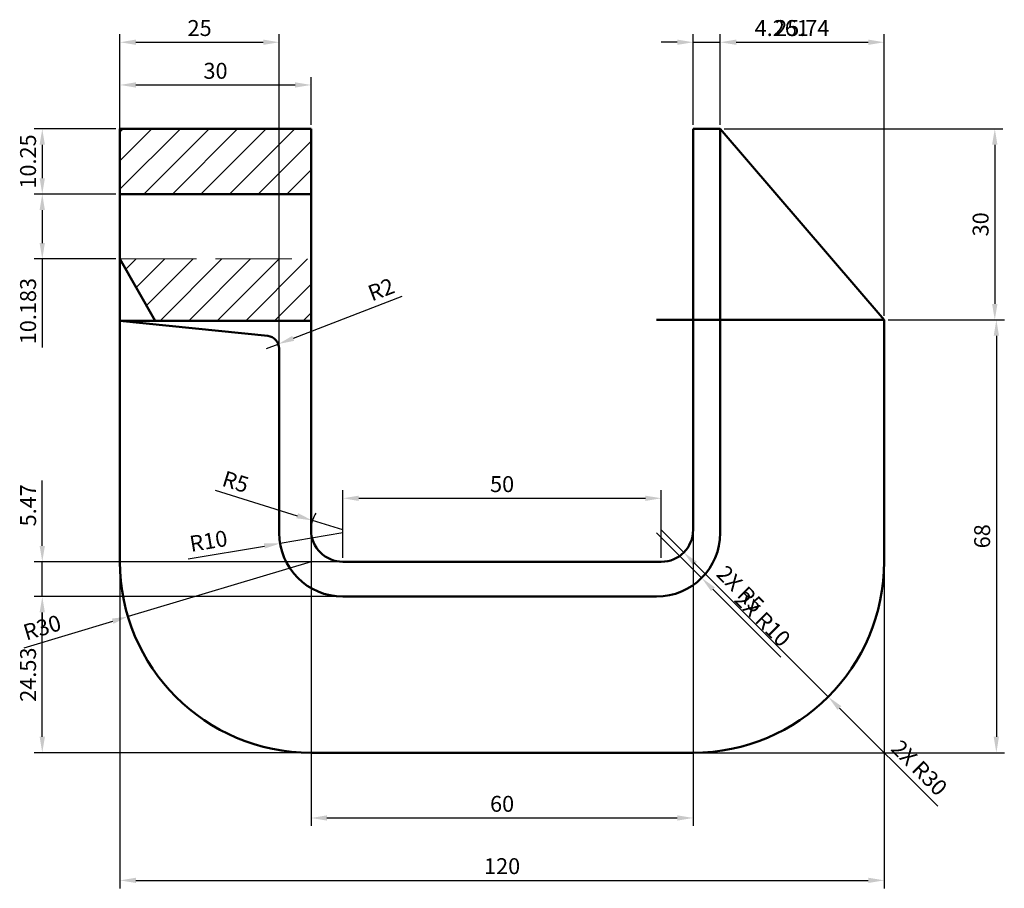
# Model space of a CAD drawing. Units: millimetres. Extents: x 1139 to 1488, y 1435 to 1756.
# Tile 2 of 3: x 1139 to 1294, y 1620 to 1756. Entities that reach past the tile are written whole.
import ezdxf

# ---------------------------------------------------------------- set-up
doc = ezdxf.new("R2010")
doc.units = ezdxf.units.MM
doc.linetypes.add('ACAD_ISO02W100', pattern=[15, 12, -3])
for name, color, linetype, lineweight in [('M-CNTR', 4, 'ACAD_ISO02W100', 18), ('M-DIMS', 2, 'Continuous', 25), ('M-HATC', 8, 'Continuous', 18), ('M-OUTL', 7, 'Continuous', 50)]:
    doc.layers.add(name, color=color, linetype=linetype, lineweight=lineweight)
doc.styles.get("Standard").update_dxf_attribs({"font": 'arial.ttf'})
doc.dimstyles.new('ISO-25', dxfattribs={"dimtxt": 2.5, "dimasz": 2.5, "dimexe": 1.25, "dimexo": 0.625, "dimtad": 1, "dimtxsty": 'Standard', "dimcen": 2.5, "dimadec": 0, "dimazin": 0, "dimtfac": 1, "dimtmove": 0, "dimatfit": 3, "dimfxl": 1, "dimarcsym": 0})

# ---------------------------------------------------------------- blocks, each defined once
blk = doc.blocks.new('*D1')
at = {"layer": 'Defpoints', "color": 0, "transparency": 16777216}
for p in [(1184.88, 1746), (1154.88, 1739.11), (1184.88, 1739.11)]:
    blk.add_point(p, dxfattribs=at)
at = {"layer": 'M-DIMS', "color": 0, "lineweight": -2, "transparency": 16777216}
for p, q in [((1154.88, 1739.73), (1154.88, 1747.25)), ((1184.88, 1739.73), (1184.88, 1747.25)), ((1157.38, 1746), (1182.38, 1746))]:
    blk.add_line(p, q, dxfattribs=at)
at = {"layer": 'M-DIMS', "color": 0, "transparency": 16777216}
for points in [[(1157.38, 1746.42), (1157.38, 1745.59), (1154.88, 1746)], [(1182.38, 1746.42), (1182.38, 1745.59), (1184.88, 1746)]]:
    blk.add_solid(points, dxfattribs=at)
at = {"layer": 'M-DIMS', "color": 0, "transparency": 16777216, "insert": (1169.88, 1747.9), "char_height": 2.5, "attachment_point": 5}
blk.add_mtext('30', dxfattribs=at)
blk = doc.blocks.new('*D2')
at = {"layer": 'Defpoints', "color": 0, "transparency": 16777216}
for p in [(1154.88, 1671.11), (1274.88, 1671.11), (1274.88, 1621.06)]:
    blk.add_point(p, dxfattribs=at)
at = {"layer": 'M-DIMS', "color": 0, "lineweight": -2, "transparency": 16777216}
for p, q in [((1154.88, 1670.48), (1154.88, 1619.81)), ((1274.88, 1670.48), (1274.88, 1619.81)), ((1157.38, 1621.06), (1272.38, 1621.06))]:
    blk.add_line(p, q, dxfattribs=at)
at = {"layer": 'M-DIMS', "color": 0, "transparency": 16777216}
for points in [[(1157.38, 1621.48), (1157.38, 1620.65), (1154.88, 1621.06)], [(1272.38, 1621.48), (1272.38, 1620.65), (1274.88, 1621.06)]]:
    blk.add_solid(points, dxfattribs=at)
at = {"layer": 'M-DIMS', "color": 0, "transparency": 16777216, "insert": (1214.88, 1622.97), "char_height": 2.5, "attachment_point": 5}
blk.add_mtext('120', dxfattribs=at)
blk = doc.blocks.new('*D3')
at = {"layer": 'Defpoints', "color": 0, "transparency": 16777216}
for p in [(1184.88, 1676.11), (1244.88, 1676.11), (1244.88, 1630.86)]:
    blk.add_point(p, dxfattribs=at)
at = {"layer": 'M-DIMS', "color": 0, "lineweight": -2, "transparency": 16777216}
for p, q in [((1184.88, 1675.48), (1184.88, 1629.61)), ((1244.88, 1675.48), (1244.88, 1629.61)), ((1187.38, 1630.86), (1242.38, 1630.86))]:
    blk.add_line(p, q, dxfattribs=at)
at = {"layer": 'M-DIMS', "color": 0, "transparency": 16777216}
for points in [[(1187.38, 1631.28), (1187.38, 1630.45), (1184.88, 1630.86)], [(1242.38, 1631.28), (1242.38, 1630.45), (1244.88, 1630.86)]]:
    blk.add_solid(points, dxfattribs=at)
at = {"layer": 'M-DIMS', "color": 0, "transparency": 16777216, "insert": (1214.88, 1632.76), "char_height": 2.5, "attachment_point": 5}
blk.add_mtext('60', dxfattribs=at)
blk = doc.blocks.new('*D4')
at = {"layer": 'Defpoints', "color": 0, "transparency": 16777216}
for p in [(1239.88, 1681.08), (1189.88, 1671.11), (1239.88, 1671.11)]:
    blk.add_point(p, dxfattribs=at)
at = {"layer": 'M-DIMS', "color": 0, "lineweight": -2, "transparency": 16777216}
for p, q in [((1189.88, 1671.73), (1189.88, 1682.33)), ((1239.88, 1671.73), (1239.88, 1682.33)), ((1192.38, 1681.08), (1237.38, 1681.08))]:
    blk.add_line(p, q, dxfattribs=at)
at = {"layer": 'M-DIMS', "color": 0, "transparency": 16777216}
for points in [[(1192.38, 1681.49), (1192.38, 1680.66), (1189.88, 1681.08)], [(1237.38, 1681.49), (1237.38, 1680.66), (1239.88, 1681.08)]]:
    blk.add_solid(points, dxfattribs=at)
at = {"layer": 'M-DIMS', "color": 0, "transparency": 16777216, "insert": (1214.88, 1682.98), "char_height": 2.5, "attachment_point": 5}
blk.add_mtext('50', dxfattribs=at)
blk = doc.blocks.new('*D5')
at = {"layer": 'Defpoints', "color": 0, "transparency": 16777216}
for p in [(1185.1, 1677.59), (1189.88, 1676.11)]:
    blk.add_point(p, dxfattribs=at)
at = {"layer": 'M-DIMS', "color": 0, "lineweight": -2, "transparency": 16777216}
for p, q in [((1169.84, 1682.34), (1182.71, 1678.33)), ((1189.88, 1676.11), (1185.1, 1677.59))]:
    blk.add_line(p, q, dxfattribs=at)
blk.add_arc((1189.88, 1676.11), 5, 148.4033, 172.838, dxfattribs=at)
at = {"layer": 'M-DIMS', "color": 0, "transparency": 16777216}
blk.add_solid([(1182.84, 1678.73), (1182.59, 1677.94), (1185.1, 1677.59)], dxfattribs=at)
at = {"layer": 'M-DIMS', "color": 0, "transparency": 16777216, "insert": (1172.94, 1683.36), "char_height": 2.5, "attachment_point": 5, "rotation": 342.7273}
blk.add_mtext('R5', dxfattribs=at)
blk = doc.blocks.new('*D6')
at = {"layer": 'Defpoints', "color": 0, "transparency": 16777216}
for p in [(1189.88, 1675.64), (1180.01, 1673.99)]:
    blk.add_point(p, dxfattribs=at)
at = {"layer": 'M-DIMS', "color": 0, "lineweight": -2, "transparency": 16777216}
for p, q in [((1189.88, 1675.64), (1180.01, 1673.99)), ((1165.58, 1671.58), (1177.55, 1673.58))]:
    blk.add_line(p, q, dxfattribs=at)
at = {"layer": 'M-DIMS', "color": 0, "transparency": 16777216}
blk.add_solid([(1177.48, 1673.99), (1177.61, 1673.17), (1180.01, 1673.99)], dxfattribs=at)
at = {"layer": 'M-DIMS', "color": 0, "transparency": 16777216, "insert": (1168.83, 1674.05), "char_height": 2.5, "attachment_point": 5, "rotation": 9.4844}
blk.add_mtext('R10', dxfattribs=at)
blk = doc.blocks.new('*D7')
at = {"layer": 'Defpoints', "color": 0, "transparency": 16777216}
for p in [(1184.88, 1671.11), (1156.14, 1662.5)]:
    blk.add_point(p, dxfattribs=at)
at = {"layer": 'M-DIMS', "color": 0, "lineweight": -2, "transparency": 16777216}
for p, q in [((1184.88, 1671.11), (1156.14, 1662.5)), ((1139.84, 1657.61), (1153.74, 1661.78))]:
    blk.add_line(p, q, dxfattribs=at)
at = {"layer": 'M-DIMS', "color": 0, "transparency": 16777216}
blk.add_solid([(1153.62, 1662.18), (1153.86, 1661.38), (1156.14, 1662.5)], dxfattribs=at)
at = {"layer": 'M-DIMS', "color": 0, "transparency": 16777216, "insert": (1142.75, 1660.47), "char_height": 2.5, "attachment_point": 5, "rotation": 16.6813}
blk.add_mtext('R30', dxfattribs=at)
blk = doc.blocks.new('*D8')
at = {"layer": 'Defpoints', "color": 0, "transparency": 16777216}
for p in [(1179.74, 1705.3), (1177.88, 1704.59)]:
    blk.add_point(p, dxfattribs=at)
at = {"layer": 'M-DIMS', "color": 0, "lineweight": -2, "transparency": 16777216}
for p, q in [((1199.13, 1712.77), (1182.07, 1706.2)), ((1177.88, 1704.59), (1179.74, 1705.3))]:
    blk.add_line(p, q, dxfattribs=at)
at = {"layer": 'M-DIMS', "color": 0, "transparency": 16777216}
blk.add_solid([(1181.93, 1706.59), (1182.22, 1705.81), (1179.74, 1705.3)], dxfattribs=at)
at = {"layer": 'M-DIMS', "color": 0, "transparency": 16777216, "insert": (1196, 1713.58), "char_height": 2.5, "attachment_point": 5, "rotation": 21.0623}
blk.add_mtext('R2', dxfattribs=at)
blk = doc.blocks.new('*D9')
at = {"layer": 'Defpoints', "color": 0, "transparency": 16777216}
for p in [(1274.88, 1709.11), (1244.88, 1641.11), (1292.49, 1641.11)]:
    blk.add_point(p, dxfattribs=at)
at = {"layer": 'M-DIMS', "color": 0, "lineweight": -2, "transparency": 16777216}
for p, q in [((1275.5, 1709.11), (1293.74, 1709.11)), ((1292.49, 1706.61), (1292.49, 1643.61)), ((1245.5, 1641.11), (1293.74, 1641.11))]:
    blk.add_line(p, q, dxfattribs=at)
at = {"layer": 'M-DIMS', "color": 0, "transparency": 16777216}
for points in [[(1292.07, 1706.61), (1292.9, 1706.61), (1292.49, 1709.11)], [(1292.07, 1643.61), (1292.9, 1643.61), (1292.49, 1641.11)]]:
    blk.add_solid(points, dxfattribs=at)
at = {"layer": 'M-DIMS', "color": 0, "transparency": 16777216, "insert": (1290.58, 1675.11), "char_height": 2.5, "attachment_point": 5, "rotation": 90}
blk.add_mtext('68', dxfattribs=at)
blk = doc.blocks.new('*D10')
at = {"layer": 'Defpoints', "color": 0, "transparency": 16777216}
for p in [(1249.14, 1739.11), (1274.88, 1709.11), (1292.24, 1709.11)]:
    blk.add_point(p, dxfattribs=at)
at = {"layer": 'M-DIMS', "color": 0, "lineweight": -2, "transparency": 16777216}
for p, q in [((1249.76, 1739.11), (1293.49, 1739.11)), ((1292.24, 1736.61), (1292.24, 1711.61)), ((1275.5, 1709.11), (1293.49, 1709.11))]:
    blk.add_line(p, q, dxfattribs=at)
at = {"layer": 'M-DIMS', "color": 0, "transparency": 16777216}
for points in [[(1291.82, 1736.61), (1292.66, 1736.61), (1292.24, 1739.11)], [(1291.82, 1711.61), (1292.66, 1711.61), (1292.24, 1709.11)]]:
    blk.add_solid(points, dxfattribs=at)
at = {"layer": 'M-DIMS', "color": 0, "transparency": 16777216, "insert": (1290.34, 1724.11), "char_height": 2.5, "attachment_point": 5, "rotation": 90}
blk.add_mtext('30', dxfattribs=at)
blk = doc.blocks.new('*D28')
at = {"layer": 'Defpoints', "color": 0, "transparency": 16777216}
for p in [(1179.88, 1752.71), (1154.88, 1708.98), (1179.88, 1704.59)]:
    blk.add_point(p, dxfattribs=at)
at = {"layer": 'M-DIMS', "color": 0, "lineweight": -2, "transparency": 16777216}
for p, q in [((1154.88, 1709.6), (1154.88, 1753.96)), ((1179.88, 1705.21), (1179.88, 1753.96)), ((1157.38, 1752.71), (1177.38, 1752.71))]:
    blk.add_line(p, q, dxfattribs=at)
at = {"layer": 'M-DIMS', "color": 0, "transparency": 16777216}
for points in [[(1157.38, 1753.13), (1157.38, 1752.3), (1154.88, 1752.71)], [(1177.38, 1753.13), (1177.38, 1752.3), (1179.88, 1752.71)]]:
    blk.add_solid(points, dxfattribs=at)
at = {"layer": 'M-DIMS', "color": 0, "transparency": 16777216, "insert": (1167.38, 1754.62), "char_height": 2.5, "attachment_point": 5}
blk.add_mtext('25', dxfattribs=at)
blk = doc.blocks.new('*D29')
at = {"layer": 'Defpoints', "color": 0, "transparency": 16777216}
for p in [(1249.14, 1752.71), (1244.88, 1739.11), (1249.14, 1739.11)]:
    blk.add_point(p, dxfattribs=at)
at = {"layer": 'M-DIMS', "color": 0, "lineweight": -2, "transparency": 16777216}
for p, q in [((1244.88, 1739.73), (1244.88, 1753.96)), ((1249.14, 1739.73), (1249.14, 1753.96)), ((1242.38, 1752.71), (1239.88, 1752.71)), ((1244.88, 1752.71), (1249.14, 1752.71)), ((1251.64, 1752.71), (1263.44, 1752.71))]:
    blk.add_line(p, q, dxfattribs=at)
at = {"layer": 'M-DIMS', "color": 0, "transparency": 16777216}
for points in [[(1242.38, 1753.13), (1242.38, 1752.3), (1244.88, 1752.71)], [(1251.64, 1753.13), (1251.64, 1752.3), (1249.14, 1752.71)]]:
    blk.add_solid(points, dxfattribs=at)
at = {"layer": 'M-DIMS', "color": 0, "transparency": 16777216, "insert": (1258.79, 1754.62), "char_height": 2.5, "attachment_point": 5}
blk.add_mtext('4.261', dxfattribs=at)
blk = doc.blocks.new('*D30')
at = {"layer": 'Defpoints', "color": 0, "transparency": 16777216}
for p in [(1274.88, 1752.71), (1249.14, 1739.11), (1274.88, 1709.11)]:
    blk.add_point(p, dxfattribs=at)
at = {"layer": 'M-DIMS', "color": 0, "lineweight": -2, "transparency": 16777216}
for p, q in [((1249.14, 1739.73), (1249.14, 1753.96)), ((1274.88, 1709.73), (1274.88, 1753.96)), ((1251.64, 1752.71), (1272.38, 1752.71))]:
    blk.add_line(p, q, dxfattribs=at)
at = {"layer": 'M-DIMS', "color": 0, "transparency": 16777216}
for points in [[(1251.64, 1753.13), (1251.64, 1752.3), (1249.14, 1752.71)], [(1272.38, 1753.13), (1272.38, 1752.3), (1274.88, 1752.71)]]:
    blk.add_solid(points, dxfattribs=at)
at = {"layer": 'M-DIMS', "color": 0, "transparency": 16777216, "insert": (1262.01, 1754.62), "char_height": 2.5, "attachment_point": 5}
blk.add_mtext('25.74', dxfattribs=at)
blk = doc.blocks.new('*D31')
at = {"layer": 'Defpoints', "color": 0, "transparency": 16777216}
for p in [(1142.68, 1665.64), (1189.88, 1665.64), (1184.88, 1641.11)]:
    blk.add_point(p, dxfattribs=at)
at = {"layer": 'M-DIMS', "color": 0, "lineweight": -2, "transparency": 16777216}
for p, q in [((1189.25, 1665.64), (1141.43, 1665.64)), ((1142.68, 1643.61), (1142.68, 1663.14)), ((1184.25, 1641.11), (1141.43, 1641.11))]:
    blk.add_line(p, q, dxfattribs=at)
at = {"layer": 'M-DIMS', "color": 0, "transparency": 16777216}
for points in [[(1142.26, 1663.14), (1143.09, 1663.14), (1142.68, 1665.64)], [(1142.26, 1643.61), (1143.09, 1643.61), (1142.68, 1641.11)]]:
    blk.add_solid(points, dxfattribs=at)
at = {"layer": 'M-DIMS', "color": 0, "transparency": 16777216, "insert": (1140.77, 1653.37), "char_height": 2.5, "attachment_point": 5, "rotation": 90}
blk.add_mtext('24.53', dxfattribs=at)
blk = doc.blocks.new('*D32')
at = {"layer": 'Defpoints', "color": 0, "transparency": 16777216}
for p in [(1142.68, 1671.11), (1189.88, 1671.11), (1189.88, 1665.64)]:
    blk.add_point(p, dxfattribs=at)
at = {"layer": 'M-DIMS', "color": 0, "lineweight": -2, "transparency": 16777216}
for p, q in [((1142.68, 1673.61), (1142.68, 1683.85)), ((1189.25, 1671.11), (1141.43, 1671.11)), ((1142.68, 1665.64), (1142.68, 1671.11)), ((1189.25, 1665.64), (1141.43, 1665.64)), ((1142.68, 1663.14), (1142.68, 1660.64))]:
    blk.add_line(p, q, dxfattribs=at)
at = {"layer": 'M-DIMS', "color": 0, "transparency": 16777216}
for points in [[(1142.26, 1673.61), (1143.09, 1673.61), (1142.68, 1671.11)], [(1142.26, 1663.14), (1143.09, 1663.14), (1142.68, 1665.64)]]:
    blk.add_solid(points, dxfattribs=at)
at = {"layer": 'M-DIMS', "color": 0, "transparency": 16777216, "insert": (1140.78, 1679.98), "char_height": 2.5, "attachment_point": 5, "rotation": 90}
blk.add_mtext('5.47', dxfattribs=at)
blk = doc.blocks.new('*D33')
at = {"layer": 'Defpoints', "color": 0, "transparency": 16777216}
for p in [(1154.88, 1739.11), (1142.68, 1728.86), (1154.88, 1728.86)]:
    blk.add_point(p, dxfattribs=at)
at = {"layer": 'M-DIMS', "color": 0, "lineweight": -2, "transparency": 16777216}
for p, q in [((1154.25, 1739.11), (1141.43, 1739.11)), ((1142.68, 1736.61), (1142.68, 1731.36)), ((1154.25, 1728.86), (1141.43, 1728.86))]:
    blk.add_line(p, q, dxfattribs=at)
at = {"layer": 'M-DIMS', "color": 0, "transparency": 16777216}
for points in [[(1142.26, 1736.61), (1143.09, 1736.61), (1142.68, 1739.11)], [(1142.26, 1731.36), (1143.09, 1731.36), (1142.68, 1728.86)]]:
    blk.add_solid(points, dxfattribs=at)
at = {"layer": 'M-DIMS', "color": 0, "transparency": 16777216, "insert": (1140.77, 1733.98), "char_height": 2.5, "attachment_point": 5, "rotation": 90}
blk.add_mtext('10.25', dxfattribs=at)
blk = doc.blocks.new('*D34')
at = {"layer": 'Defpoints', "color": 0, "transparency": 16777216}
for p in [(1154.88, 1728.86), (1142.68, 1718.67), (1154.88, 1718.67)]:
    blk.add_point(p, dxfattribs=at)
at = {"layer": 'M-DIMS', "color": 0, "lineweight": -2, "transparency": 16777216}
for p, q in [((1154.25, 1728.86), (1141.43, 1728.86)), ((1142.68, 1726.36), (1142.68, 1721.17)), ((1154.25, 1718.67), (1141.43, 1718.67)), ((1142.68, 1718.67), (1142.68, 1704.78))]:
    blk.add_line(p, q, dxfattribs=at)
at = {"layer": 'M-DIMS', "color": 0, "transparency": 16777216}
for points in [[(1142.26, 1726.36), (1143.09, 1726.36), (1142.68, 1728.86)], [(1142.26, 1721.17), (1143.09, 1721.17), (1142.68, 1718.67)]]:
    blk.add_solid(points, dxfattribs=at)
at = {"layer": 'M-DIMS', "color": 0, "transparency": 16777216, "insert": (1140.77, 1710.48), "char_height": 2.5, "attachment_point": 5, "rotation": 90}
blk.add_mtext('10.183', dxfattribs=at)
blk = doc.blocks.new('*D51')
at = {"layer": 'Defpoints', "color": 0, "transparency": 16777216}
for p in [(1244.88, 1671.11), (1266.09, 1649.89)]:
    blk.add_point(p, dxfattribs=at)
at = {"layer": 'M-DIMS', "color": 0, "lineweight": -2, "transparency": 16777216}
for p, q in [((1244.88, 1671.11), (1266.09, 1649.89)), ((1283.28, 1632.7), (1267.86, 1648.13))]:
    blk.add_line(p, q, dxfattribs=at)
at = {"layer": 'M-DIMS', "color": 0, "transparency": 16777216}
blk.add_solid([(1268.15, 1648.42), (1267.56, 1647.83), (1266.09, 1649.89)], dxfattribs=at)
at = {"layer": 'M-DIMS', "color": 0, "transparency": 16777216, "insert": (1280.16, 1638.51), "char_height": 2.5, "attachment_point": 5, "rotation": 315.0007}
blk.add_mtext('2X R30', dxfattribs=at)
blk = doc.blocks.new('*D52')
at = {"layer": 'Defpoints', "color": 0, "transparency": 16777216}
for p in [(1239.14, 1675.64), (1246.21, 1668.57)]:
    blk.add_point(p, dxfattribs=at)
at = {"layer": 'M-DIMS', "color": 0, "lineweight": -2, "transparency": 16777216}
for p, q in [((1239.14, 1675.64), (1246.21, 1668.57)), ((1258.67, 1656.1), (1247.98, 1666.8))]:
    blk.add_line(p, q, dxfattribs=at)
at = {"layer": 'M-DIMS', "color": 0, "transparency": 16777216}
blk.add_solid([(1248.27, 1667.09), (1247.68, 1666.5), (1246.21, 1668.57)], dxfattribs=at)
at = {"layer": 'M-DIMS', "color": 0, "transparency": 16777216, "insert": (1255.55, 1661.91), "char_height": 2.5, "attachment_point": 5, "rotation": 315.0005}
blk.add_mtext('2X R10', dxfattribs=at)
blk = doc.blocks.new('*D53')
at = {"layer": 'Defpoints', "color": 0, "transparency": 16777216}
for p in [(1239.88, 1676.11), (1243.41, 1672.57)]:
    blk.add_point(p, dxfattribs=at)
at = {"layer": 'M-DIMS', "color": 0, "lineweight": -2, "transparency": 16777216}
for p, q in [((1239.88, 1676.11), (1243.41, 1672.57)), ((1254.52, 1661.46), (1245.18, 1670.8))]:
    blk.add_line(p, q, dxfattribs=at)
at = {"layer": 'M-DIMS', "color": 0, "transparency": 16777216}
blk.add_solid([(1245.47, 1671.1), (1244.88, 1670.51), (1243.41, 1672.57)], dxfattribs=at)
at = {"layer": 'M-DIMS', "color": 0, "transparency": 16777216, "insert": (1252.08, 1666.59), "char_height": 2.5, "attachment_point": 5, "rotation": 314.9963}
blk.add_mtext('2X R5', dxfattribs=at)

msp = doc.modelspace()

# ---------------------------------------------------------------- hatches: boundary and pattern name
at = {"layer": 'M-HATC'}
h = msp.add_hatch(dxfattribs=at)
h.set_pattern_fill('ANSI31', color=256)
h.paths.add_polyline_path([(1154.8755, 1739.107), (1154.8755, 1728.8567), (1184.8755, 1728.8567), (1184.8755, 1739.107)])
h.paths.add_polyline_path([(1184.8755, 1708.9759), (1184.8755, 1718.6734), (1154.8755, 1718.6734), (1160.4078, 1708.9759)])

# ---------------------------------------------------------------- linework, layer by layer
at = {"layer": 'M-CNTR'}
msp.add_line((1154.8755, 1718.6734), (1184.8755, 1718.6734), dxfattribs=at)
at = {"layer": 'M-OUTL'}
for p, q in [((1154.8755, 1671.107), (1154.8755, 1739.107)), ((1154.8755, 1739.107), (1184.8755, 1739.107)), ((1184.8755, 1739.107), (1179.8755, 1739.107)), ((1184.8755, 1739.107), (1184.8755, 1708.9759)), ((1249.1366, 1739.107), (1244.8755, 1739.107)), ((1244.8755, 1739.107), (1244.8755, 1676.107)), ((1249.1366, 1739.107), (1249.1366, 1675.6373)), ((1249.1366, 1739.107), (1274.8755, 1709.107)), ((1154.8755, 1728.8567), (1184.8755, 1728.8567)), ((1154.8755, 1718.6734), (1160.4078, 1708.9759)), ((1154.8755, 1708.9759), (1184.8755, 1708.9759)), ((1154.8755, 1708.9759), (1178.0813, 1706.5751)), ((1184.8755, 1705.8722), (1184.8755, 1708.9759)), ((1274.8755, 1709.107), (1239.115, 1709.107)), ((1274.8755, 1671.107), (1274.8755, 1709.107)), ((1184.8755, 1705.8722), (1184.8755, 1676.107)), ((1179.8755, 1704.5857), (1179.8755, 1675.6373)), ((1239.8755, 1671.107), (1189.8755, 1671.107)), ((1239.1366, 1665.6373), (1189.8755, 1665.6373)), ((1184.8755, 1641.107), (1244.8755, 1641.107))]:
    msp.add_line(p, q, dxfattribs=at)
for centre, radius, start, end in [((1177.8755, 1704.5857), 2, 360, 84.093551), ((1189.8755, 1676.107), 5, 180, 270), ((1239.8755, 1676.107), 5, 270, 0), ((1189.8755, 1675.6373), 10, 180, 270), ((1239.1366, 1675.6373), 10, 270, 0), ((1184.8755, 1671.107), 30, 180, 270), ((1244.8755, 1671.107), 30, 270, 0)]:
    msp.add_arc(centre, radius, start, end, dxfattribs=at)

# ---------------------------------------------------------------- dimensions: what is measured, and where the dimension line sits
at = {"layer": 'M-DIMS'}
for base, p1, p2, override, picture, middle in [((1179.8755, 1752.714), (1154.8755, 1708.9759), (1179.8755, 1704.5857), {"dimdec": 0, "dimlfac": 1, "dimrnd": 0, "dimzin": 0, "dimdsep": 46, "dimlunit": 2}, '*D28', (1167.3755, 1754.6154)), ((1249.1366, 1752.714), (1244.8755, 1739.107), (1249.1366, 1739.107), {"dimdec": 3, "dimlfac": 1, "dimrnd": 0, "dimzin": 0, "dimdsep": 46, "dimlunit": 2}, '*D29', (1258.7887, 1754.6154)), ((1274.8755, 1752.714), (1249.1366, 1739.107), (1274.8755, 1709.107), {"dimdec": 2, "dimlfac": 1, "dimrnd": 0, "dimzin": 0, "dimdsep": 46, "dimlunit": 2}, '*D30', (1262.006, 1754.6154)), ((1184.8755, 1746.0023), (1154.8755, 1739.107), (1184.8755, 1739.107), {"dimclrd": 0, "dimclre": 0, "dimclrt": 0}, '*D1', (1169.8755, 1747.9046)), ((1239.8755, 1681.0776), (1189.8755, 1671.107), (1239.8755, 1671.107), {"dimclrd": 0, "dimclre": 0, "dimclrt": 0}, '*D4', (1214.8755, 1682.979)), ((1244.8755, 1630.8625), (1184.8755, 1676.107), (1244.8755, 1676.107), {"dimclrd": 0, "dimclre": 0, "dimclrt": 0}, '*D3', (1214.8755, 1632.7639)), ((1274.8755, 1621.0644), (1154.8755, 1671.107), (1274.8755, 1671.107), {"dimclrd": 0, "dimclre": 0, "dimclrt": 0}, '*D2', (1214.8755, 1622.9658))]:
    dim = msp.add_linear_dim(base=base, p1=p1, p2=p2, dimstyle='ISO-25', override=override, dxfattribs=at)
    dim.commit()
    dim.dimension.update_dxf_attribs({"geometry": picture, "text_midpoint": middle})
for base, p1, p2, override, picture, middle in [((1142.6755, 1728.8567), (1154.8755, 1739.107), (1154.8755, 1728.8567), {"dimdec": 2, "dimlfac": 1, "dimrnd": 0, "dimzin": 0, "dimdsep": 46, "dimlunit": 2}, '*D33', (1140.774, 1733.9819)), ((1292.2395, 1709.107), (1249.1366, 1739.107), (1274.8755, 1709.107), {"dimclrd": 0, "dimclre": 0, "dimclrt": 0}, '*D10', (1290.3372, 1724.107)), ((1142.6755, 1718.6734), (1154.8755, 1728.8567), (1154.8755, 1718.6734), {"dimdec": 3, "dimlfac": 1, "dimrnd": 0, "dimzin": 0, "dimdsep": 46, "dimlunit": 2}, '*D34', (1140.7732, 1710.4768)), ((1292.4855, 1641.107), (1274.8755, 1709.107), (1244.8755, 1641.107), {"dimclrd": 0, "dimclre": 0, "dimclrt": 0}, '*D9', (1290.5841, 1675.107)), ((1142.6755, 1671.107), (1189.8755, 1665.6373), (1189.8755, 1671.107), {"dimdec": 2, "dimlfac": 1, "dimrnd": 0, "dimzin": 0, "dimdsep": 46, "dimlunit": 2}, '*D32', (1140.7791, 1679.9789)), ((1142.6755, 1665.6373), (1184.8755, 1641.107), (1189.8755, 1665.6373), {"dimdec": 2, "dimlfac": 1, "dimrnd": 0, "dimzin": 0, "dimdsep": 46, "dimlunit": 2}, '*D31', (1140.7732, 1653.3721))]:
    dim = msp.add_linear_dim(base=base, p1=p1, p2=p2, angle=90, dimstyle='ISO-25', override=override, dxfattribs=at)
    dim.commit()
    dim.dimension.update_dxf_attribs({"geometry": picture, "text_midpoint": middle})
for center, mpoint, picture, middle in [((1177.8755, 1704.5857), (1179.7418, 1705.3045), '*D8', (1196.6787, 1711.8271)), ((1189.8755, 1676.107), (1185.101, 1677.5916), '*D5', (1172.3735, 1681.5491)), ((1189.8755, 1675.6373), (1180.0122, 1673.9895), '*D6', (1169.1431, 1672.1737)), ((1184.8755, 1671.107), (1156.138, 1662.4956), '*D7', (1143.2997, 1658.6485))]:
    dim = msp.add_radius_dim(center=center, mpoint=mpoint, dimstyle='ISO-25', override={"dimclrd": 0, "dimclre": 0, "dimclrt": 0}, dxfattribs=at)
    dim.commit()
    dim.dimension.update_dxf_attribs({"geometry": picture, "text_midpoint": middle, "dimtype": 164})
for center, mpoint, picture, middle in [((1239.8755, 1676.107), (1243.4108, 1672.5712), '*D53', (1252.0786, 1666.5915)), ((1239.1366, 1675.6373), (1246.2077, 1668.5663), '*D52', (1255.5531, 1661.9101))]:
    dim = msp.add_radius_dim(center=center, mpoint=mpoint, text='2X <>', dimstyle='ISO-25', override={"dimdec": 0, "dimlfac": 1, "dimrnd": 0, "dimzin": 0, "dimdsep": 46, "dimlunit": 2}, dxfattribs=at)
    dim.commit()
    dim.dimension.update_dxf_attribs({"geometry": picture, "text_midpoint": middle})
dim = msp.add_radius_dim(center=(1244.8755, 1671.107), mpoint=(1266.0889, 1649.8941), text='2X <>', dimstyle='ISO-25', override={"dimdec": 0, "dimlfac": 1, "dimrnd": 0, "dimzin": 0, "dimdsep": 46, "dimlunit": 2}, dxfattribs=at)
dim.commit()
dim.dimension.update_dxf_attribs({"geometry": '*D51', "text_midpoint": (1278.817, 1637.1663), "dimtype": 164})

doc.saveas('drawing.dxf')
